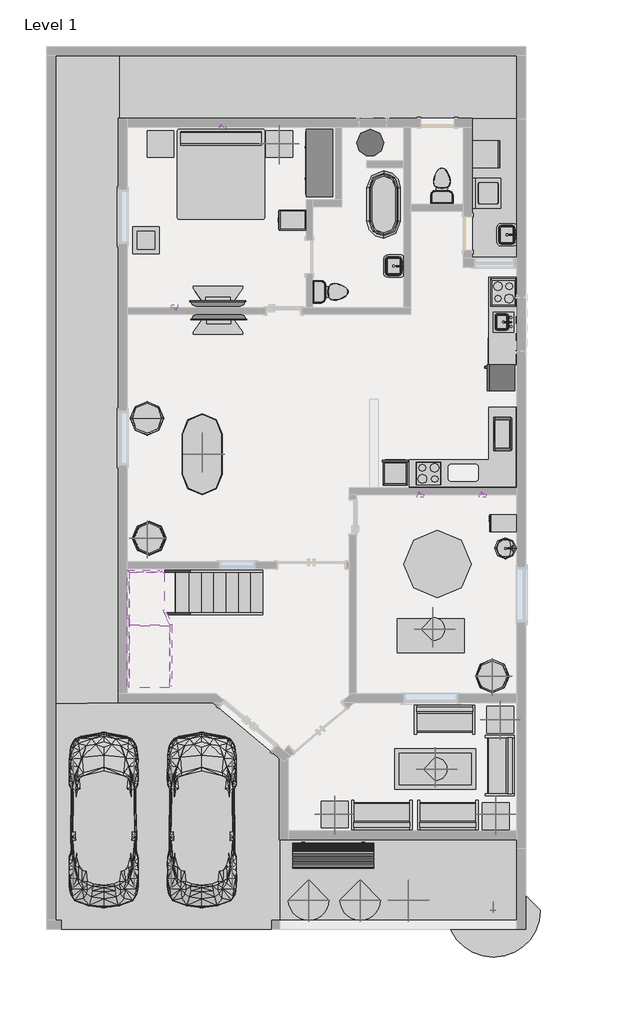
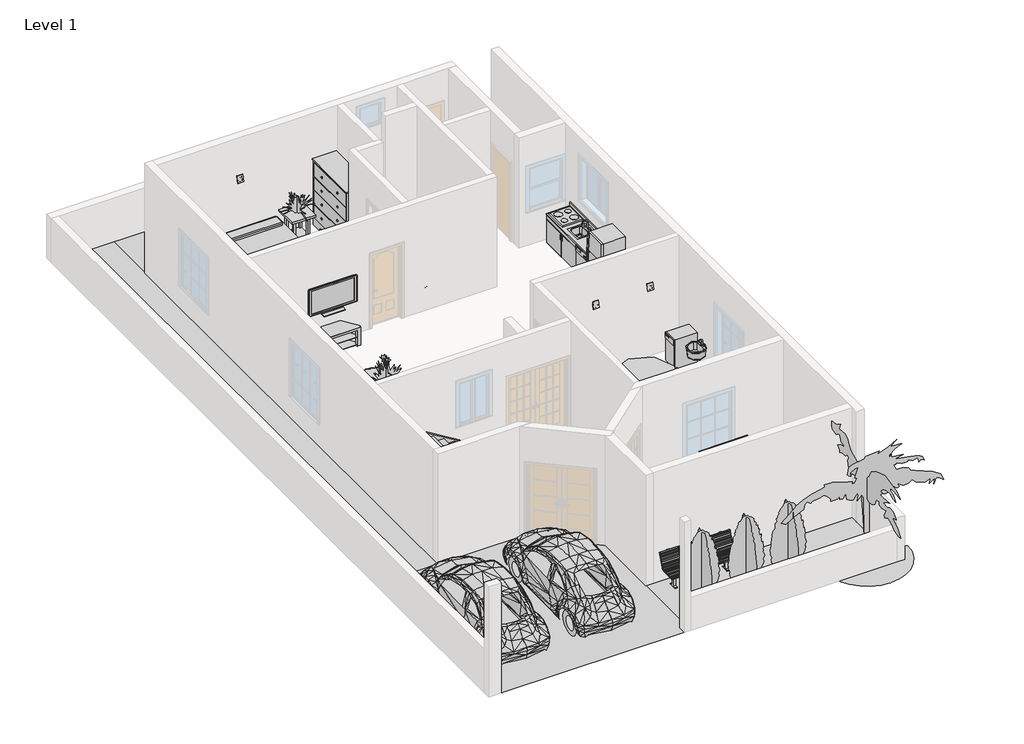
# One storey, part 2 of 2: 26 furniture elements, 21 proxies, 14 geographic elements, 8 flow terminals, 7 members, 2 stair flights, 1 slab.
# Revit data of these elements (continued)
# Element 31 (IfcFurniture, "Bed-Standard.0001 : King 78\" x 80\"")
#   Phase Created = New Construction
#   Materials on its faces: "Linen, White", "Steel, Chrome Plated"
# Element 32 (IfcFurniture, "Counter Top w Sink Hole : 24\" Depth")
#   Sink Opening Depth = 1' - 2"
#   Sink Location To Wall = 0' - 6"
#   Length = 6' - 6"
#   Sink Location = 3' - 4"
#   Sink Opening Width = 1' - 4"
#   Phase Created = New Construction
#   Materials on its faces: "Counter Top"
# Element 33 (IfcFurniture, "Counter Top-L Shaped w Sink Hole : 24\" Depth")
#   Sink Opening Width = 2' - 3"
#   Sink Opening Depth = 1' - 3"
#   Sink Location To Wall = 0' - 6"
#   Sink Location = 2' - 10 1/2"
#   Length - Leg 2 = 6' - 0"
#   Length - Leg 1 = 8' - 0"
#   Phase Created = New Construction
#   Materials on its faces: "Counter Top"
# Element 34 (IfcFurniture, "Dresser : 48\" x 72\" x 24\"")
#   Phase Created = New Construction
#   Materials on its faces: "Laminate, Ivory, Matte", "Cherry", "Laminate - Ivory, Glossy"
# Elements 35, 36, 37, 38 (IfcFurniture, "Sofa : 54\"")
#   Phase Created = New Construction
#   Materials on its faces: "Cherry"
# Elements 39, 40 (IfcFurniture, "TV - Flat Screen : 50\"")
#   Stand = yes
#   Phase Created = New Construction
#   Materials on its faces: "TV - Black", "TV - Glass", "TV - Screen"
# Elements 41, 42 (IfcFurniture, "TV Stand : TV Stand")
#   Phase Created = New Construction
#   Materials on its faces: "Melamine - Gray", "Glass - Shelves"
# Element 43 (IfcFurniture, "Table-Coffee : 24\" x 24\" x 24\"")
#   Phase Created = New Construction
#   Materials on its faces: "Glass - Clear, Grey"
# Element 44 (IfcFurniture, "Table-Coffee : 36\" x 72\" x 18\"")
#   Phase Created = New Construction
#   Materials on its faces: "Wood - Teak", "Steel, Chrome Plated", "Glass - Clear, Grey"
# Element 45 (IfcFurniture, "Table-Dining : 30\" x 84\" x 22\"")
#   Phase Created = New Construction
#   Materials on its faces: "Steel, Chrome Plated", "Glass - Clear, Grey"
# Element 46 (IfcFurniture, "Table-Dining Oval : 36\" x 72\"")
#   Phase Created = New Construction
#   Materials on its faces: "Steel, Chrome Plated", "Glass - Clear, Grey"
# Element 47 (IfcFurniture, "Table-Dining Round w Chairs : 60\" Diameter")
#   Phase Created = New Construction
#   Materials on its faces: "Pine", "Laminate, Linen, Matte"
# Elements 48, 49, 50, 51, 52 (IfcFurniture, "Table-Night Stand : 24\" x 24\" x 30\"")
#   Phase Created = New Construction
#   Materials on its faces: "Birch", "Laminate, Ivory, Matte"
# Elements 53, 54, 55 (IfcFurniture, "Table-Round : 36\" Diameter")
#   Phase Created = New Construction
#   Materials on its faces: "Steel, Chrome Plated", "Birch"
# Element 56 (IfcGeographicElement, "Park Bench : 72\"")
#   Phase Created = New Construction
#   Materials on its faces: "Wood - Teak", "Steel, Paint Finish, Dark Gray, Matte"
# Elements 57, 58, 59 (IfcGeographicElement, "RPC Plant - Tropical")
#   Phase Created = New Construction
# Elements 60, 61, 62, 63 (IfcGeographicElement, "RPC Plant - Tropical : Agave - 1.5'")
#   Phase Created = New Construction
# Elements 64, 65 (IfcGeographicElement, "RPC Plant - Tropical : Dagger - 2'")
#   Phase Created = New Construction
# Elements 66, 67, 68 (IfcGeographicElement, "RPC Tree - Conifer : Chinese Juniper - 7'")
#   Phase Created = New Construction
# Element 69 (IfcGeographicElement, "RPC Tree - Tropical : Australian Tree Furn - 6'")
#   Phase Created = New Construction
# Elements 70, 71, 72, 73, 74, 75, 76 (IfcMember, "Stringer - 2\" Width")
#   Phase Created = New Construction
# Element 77 (IfcSlab, "Non-Monolithic Landing")
#   Phase Created = New Construction
# Elements 78, 79 (IfcStairFlight, "2\" Tread 1\" Nosing 1/4\" Riser")
#   Phase Created = New Construction
# Materials
#   "Plastic, Opaque Black": class "Plastic", colour RGB 0 0 0, transparency 0.7, Description = "Plastic, generic, opaque black", Cost = 0
#   "Steel, Paint Finish, Ivory, Matte": class "Metal", colour RGB 247 247 239, transparency 0, Description = "Steel, paint finish, ivory, matte", Cost = 0
#   "Steel, Chrome Plated": class "Metal", colour RGB 17 17 17, transparency 0, Description = "Chromiuim plated steel", Cost = 0
#   "Steel, Polished": class "Metal", colour RGB 57 57 57, transparency 0, Description = "Polished steel", Cost = 0
#   "Steel, Paint Finish, Ivory, Glossy": class "Metal", colour RGB 247 247 239, transparency 0, Description = "Steel, paint finish, ivory, glossy", Cost = 0
#   "Cabinets": colour RGB 249 249 249, transparency 0
#   "Cabinets - Handles": class "Metal", colour RGB 57 57 57, transparency 0
#   "Laminate, Ivory, Matte": class "Plastic", colour RGB 247 247 239, transparency 0, Description = "Plastic Laminate - Ivory, Matte", Cost = 0
#   "Metal - Stainless Steel, Polished": class "Metal", colour RGB 216 216 216, transparency 0
#   "Porcelain, Linen": class "Ceramic", colour RGB 249 239 230, transparency 0, Description = "Porcelain, linen", Cost = 0
#   "Laminate, Linen, Matte": class "Plastic", colour RGB 249 239 230, transparency 0, Description = "Plastic Laminate - Linen, Matte", Cost = 0
#   "Porcelain, Ivory": class "Ceramic", colour RGB 247 247 239, transparency 0, Description = "Porcelain, ivory", Cost = 0
#   "Linen, White": class "Textile", colour RGB 247 247 239, transparency 0, Description = "Linen, white", Cost = 0
#   "Laminate - Ivory, Glossy": colour RGB 247 247 239, transparency 0
#   "Cherry": class "Wood", colour RGB 226 177 128, transparency 0, Description = "Prunus Serotina", Cost = 0
#   "Melamine - Gray": class "Wood", colour RGB 49 49 49, transparency 0
#   "Wood - Teak": class "Wood", colour RGB 120 73 19, transparency 0
#   "Glass - Clear, Grey": class "Glass", colour RGB 252 255 255, transparency 0.64
#   "Pine": class "Wood", colour RGB 223 192 134, transparency 0, Description = "Pinus Echinata", Cost = 0
#   "Birch": class "Wood", colour RGB 224 178 126, transparency 0, Description = "Betula Alleghaniensis", Cost = 0
#   "Steel, Paint Finish, Dark Gray, Matte": class "Metal", colour RGB 98 98 98, transparency 0, Description = "Steel, paint finish, dark gray, matte", Cost = 0
#   "Glass": class "Glass", colour RGB 0 128 192, transparency 0.75, Description = "Soda Lime Glass", Cost = 0
#   "Steel": class "Metal", colour RGB 247 247 247, transparency 0, Description = "Steel, mill finish", Cost = 0
#   "Cabinets - Panel/Glass": colour RGB 252 255 255, transparency 0.72
#   "Counter Top": class "Wood", colour RGB 226 177 128, transparency 0
#   "TV - Black": colour RGB 49 49 49, transparency 0
#   "TV - Glass": colour RGB 157 157 157, transparency 0.9
#   "TV - Screen": colour RGB 0 0 0, transparency 0
#   "Glass - Shelves": class "Glass", colour RGB 167 167 167, transparency 0.9
